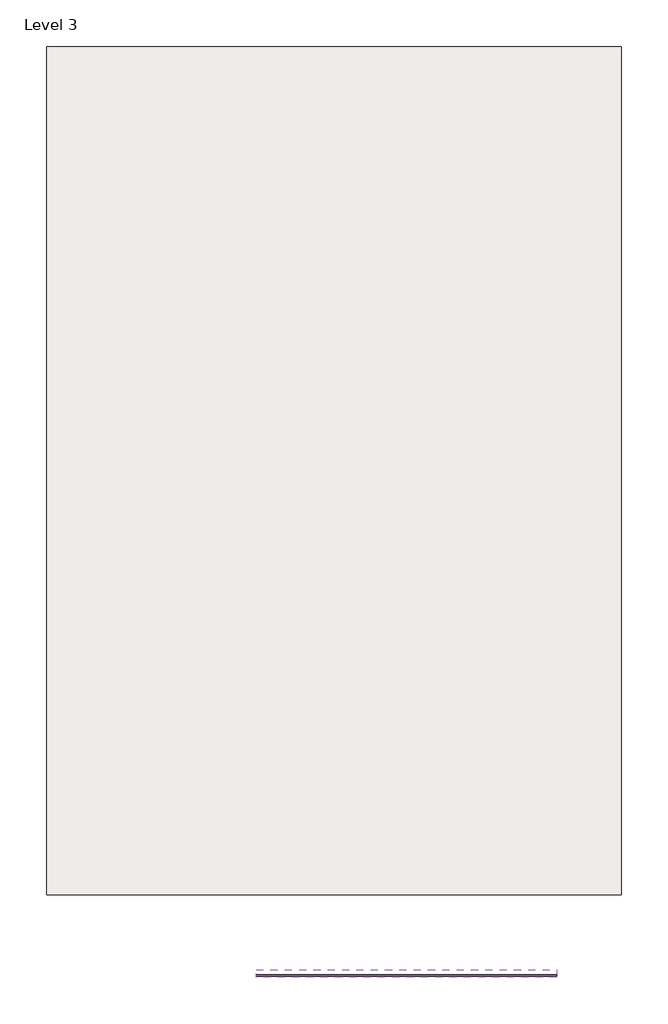
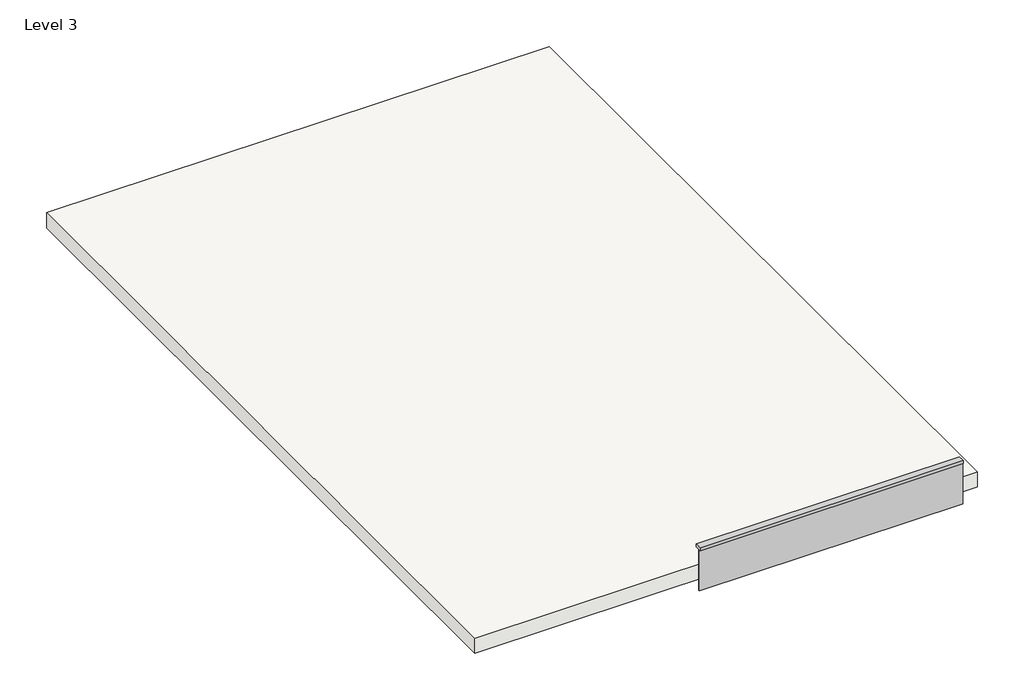
# One storey: 1 member, 1 plate, 1 roof.
"""IFC4 building model written with IfcOpenShell, lengths in millimetres."""

from ifc_helpers import new_model, si_unit, frame, origin, place, context, project, spatial, polyline, outline, extrude, transform, mapped, element, save
from components import member_94311e20, system_panel_glazed_c5f16bad

model = new_model("IFC4")

# Units and contexts
model_context = context("Model", 3, world=origin())
ifc_project = project(units=[si_unit("LENGTHUNIT", "METRE", prefix="MILLI")], contexts=[model_context])

# Site, building, storey
site = spatial("IfcSite", under=ifc_project)
building = spatial("IfcBuilding", under=site)
storey = spatial("IfcBuildingStorey", under=building, Name="Level 3", Elevation=6096.0)

# Member
placement = place(None, origin())
member_shape = member_94311e20(model_context)
element("IfcMember", 1, ObjectType="Rectangular Mullion : 2.5\" x 5\" rectangular", at=placement, inside=storey, context=model_context, shape_type="MappedRepresentation", body=[
    mapped(member_shape, transform((-15131.8718674, -16065.8200166, 7843.287052), x_axis=(0.0, 0.0, 1.0), y_axis=(0.0, 1.0, 0.0), z_axis=(-1.0, 0.0, 0.0))),
])

# Plate
system_panel_glazed_shape = system_panel_glazed_c5f16bad(model_context)
element("IfcPlate", 2, ObjectType="System Panel : Glazed", at=placement, inside=storey, context=model_context, shape_type="MappedRepresentation", body=[
    mapped(system_panel_glazed_shape, transform((-12617.2718674, -16065.8200166, 6955.069049), x_axis=(-1.0, 0.0, 0.0), y_axis=(0.0, -1.0, 0.0), z_axis=(0.0, 0.0, 1.0))),
])

# Roof
element("IfcRoof", 3, ObjectType="Generic - 12\"", at=placement, inside=storey, context=model_context, shape_type="SweptSolid", body=[
    extrude(outline(polyline([(-18633.0094994, -570.4805842), (-9031.8094994, -570.4805842), (-9031.8094994, -14743.6805842), (-18633.0094994, -14743.6805842), (-18633.0094994, -570.4805842)])), frame((0.0, 0.0, 6096.0), z_axis=(0.0, 0.0, 1.0), x_axis=(1.0, 0.0, 0.0)), (0.0, 0.0, 1.0), 304.8),
])

save(model, "model.ifc")

# Revit data of these elements
# Type "Rectangular Mullion : 2.5\" x 5\" rectangular"
#   built-in parameter 1007304 = 0.416667 (stored number, unit not read)
#   built-in parameter 1007301 = 0.104167 (stored number, unit not read)
#   built-in parameter 1007300 = 0.104167 (stored number, unit not read)
# Type "System Panel : Glazed"
#   Construction Type Id = "GSP4R"
#   Analytic Construction = "1/8 in Pilkington single glazing"
#   Visual Light Transmittance = 0.9
#   Solar Heat Gain Coefficient = 0.86
#   Heat Transfer Coefficient (U) = 1.18115 BTU/(h·ft²·°F)
#   Define Thermal Properties by = 1
# Type "Generic - 12\""
#   Assembly Code = "B1020"
#   Layers, outside or top first: 1' - 0" no material (function 1)
# Element 1 (IfcMember, "Rectangular Mullion : 2.5\" x 5\" rectangular")
#   Phase Created = New Construction
#   Materials on its faces: "Aluminum"
# Element 2 (IfcPlate, "System Panel : Glazed")
#   Phase Created = New Construction
#   Materials on its faces: "Glass"
# Element 3 (IfcRoof, "Generic - 12\"")
#   built-in parameter 1001705 = 21 (stored number, unit not read)
#   built-in parameter 1001710 = 33615
#   Phase Created = New Construction
#   Materials on its faces: "Default Roof"
# Materials
#   "Aluminum": class "Metal", colour RGB 247 247 247, transparency 0, Description = "Aluminum 6061", Cost = 0
#   "Glass": class "Glass", colour RGB 0 128 192, transparency 0.75, Description = "Soda Lime Glass", Cost = 0
#   "Default Roof": colour RGB 88 101 114, transparency 0, Cost = 0
